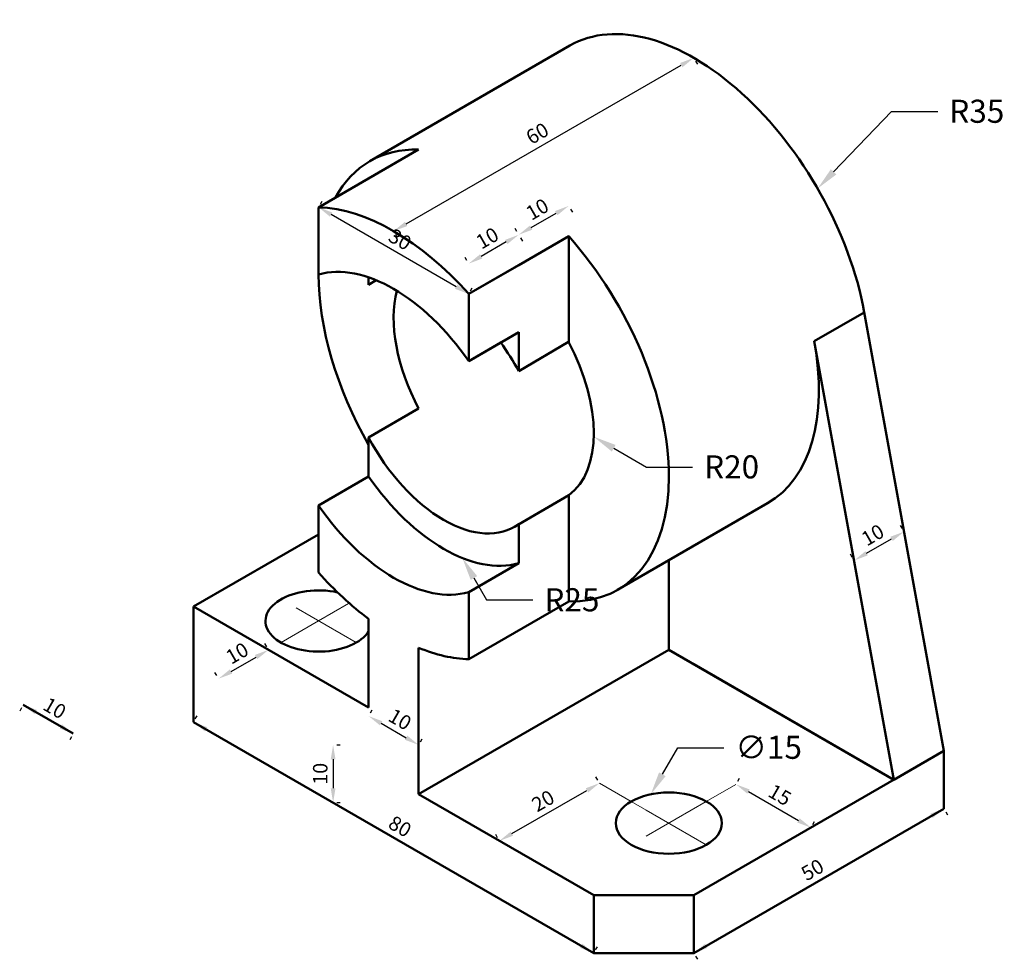
# Model space of a CAD drawing. Units: millimetres. Extents: x 7448 to 7618, y 7987 to 8150.
import ezdxf
from ezdxf import colors
from ezdxf.entities.mleader import LeaderData, LeaderLine
from ezdxf.math import Vec2, Vec3

# ---------------------------------------------------------------- set-up
doc = ezdxf.new("R2010")
doc.units = ezdxf.units.MM
doc.linetypes.add('ACAD_ISO02W100', pattern=[15, 12, -3])
for name, color, linetype, lineweight in [('M-CNTR', 1, 'ACAD_ISO02W100', 18), ('M-CONS', 8, 'ACAD_ISO02W100', 13), ('M-DIMS', 2, 'Continuous', 25), ('M-OUTL', 7, 'Continuous', 50), ('M-TEXT', 3, 'Continuous', 25)]:
    doc.layers.add(name, color=color, linetype=linetype, lineweight=lineweight)
doc.styles.get("Standard").update_dxf_attribs({"font": 'arial.ttf'})
doc.dimstyles.new('ISO-25', dxfattribs={"dimtxt": 2.5, "dimasz": 2.5, "dimexe": 1.25, "dimexo": 0.625, "dimtad": 1, "dimtxsty": 'Standard', "dimcen": 2.5, "dimadec": 0, "dimazin": 0, "dimtfac": 1, "dimtmove": 0, "dimatfit": 3, "dimfxl": 1, "dimarcsym": 0})

# ---------------------------------------------------------------- blocks, each defined once
blk = doc.blocks.new('*D1')
at = {"layer": 'Defpoints', "color": 0, "transparency": 16777216}
for p in [(7502.21, 8024.15), (7502.21, 8014.15), (7502.21, 8014.15)]:
    blk.add_point(p, dxfattribs=at)
at = {"layer": 'M-DIMS', "color": 0, "lineweight": -2, "transparency": 16777216}
for p, q in [((7502.84, 8024.15), (7503.46, 8024.15)), ((7502.21, 8021.65), (7502.21, 8016.65)), ((7502.84, 8014.15), (7503.46, 8014.15))]:
    blk.add_line(p, q, dxfattribs=at)
at = {"layer": 'M-DIMS', "color": 0, "transparency": 16777216}
for points in [[(7501.8, 8021.65), (7502.63, 8021.65), (7502.21, 8024.15)], [(7501.8, 8016.65), (7502.63, 8016.65), (7502.21, 8014.15)]]:
    blk.add_solid(points, dxfattribs=at)
at = {"layer": 'M-DIMS', "color": 0, "transparency": 16777216, "insert": (7500.31, 8019.15), "char_height": 2.5, "attachment_point": 5, "rotation": 90}
blk.add_mtext('10', dxfattribs=at)
blk = doc.blocks.new('*D2')
at = {"layer": 'Defpoints', "color": 0, "transparency": 16777216}
for p in [(7508.36, 8029.14), (7517.02, 8024.14), (7517.02, 8024.14)]:
    blk.add_point(p, dxfattribs=at)
at = {"layer": 'M-DIMS', "color": 0, "lineweight": -2, "transparency": 16777216}
for p, q in [((7508.67, 8029.68), (7508.98, 8030.22)), ((7510.52, 8027.89), (7514.85, 8025.39)), ((7517.33, 8024.68), (7517.64, 8025.22))]:
    blk.add_line(p, q, dxfattribs=at)
at = {"layer": 'M-DIMS', "color": 0, "transparency": 16777216}
for points in [[(7510.73, 8028.25), (7510.32, 8027.53), (7508.36, 8029.14)], [(7515.06, 8025.75), (7514.65, 8025.03), (7517.02, 8024.14)]]:
    blk.add_solid(points, dxfattribs=at)
at = {"layer": 'M-DIMS', "color": 0, "transparency": 16777216, "insert": (7513.64, 8028.29), "char_height": 2.5, "attachment_point": 5, "rotation": 330}
blk.add_mtext('10', dxfattribs=at)
blk = doc.blocks.new('*D3')
at = {"layer": 'Defpoints', "color": 0, "transparency": 16777216}
for p in [(7543, 8117.48), (7543, 8117.48), (7534.34, 8112.48)]:
    blk.add_point(p, dxfattribs=at)
at = {"layer": 'M-DIMS', "color": 0, "lineweight": -2, "transparency": 16777216}
for p, q in [((7543.31, 8116.93), (7543.63, 8116.39)), ((7536.51, 8113.73), (7540.84, 8116.23)), ((7534.65, 8111.93), (7534.97, 8111.39))]:
    blk.add_line(p, q, dxfattribs=at)
at = {"layer": 'M-DIMS', "color": 0, "transparency": 16777216}
for points in [[(7540.63, 8116.59), (7541.04, 8115.86), (7543, 8117.48)], [(7536.3, 8114.09), (7536.71, 8113.36), (7534.34, 8112.48)]]:
    blk.add_solid(points, dxfattribs=at)
at = {"layer": 'M-DIMS', "color": 0, "transparency": 16777216, "insert": (7537.72, 8116.62), "char_height": 2.5, "attachment_point": 5, "rotation": 30}
blk.add_mtext('10', dxfattribs=at)
blk = doc.blocks.new('*D4')
at = {"layer": 'Defpoints', "color": 0, "transparency": 16777216}
for p in [(7534.34, 8112.48), (7525.68, 8107.48), (7525.68, 8107.48)]:
    blk.add_point(p, dxfattribs=at)
at = {"layer": 'M-DIMS', "color": 0, "lineweight": -2, "transparency": 16777216}
for p, q in [((7534.03, 8113.02), (7533.72, 8113.56)), ((7532.18, 8111.23), (7527.84, 8108.73)), ((7525.37, 8108.02), (7525.05, 8108.56))]:
    blk.add_line(p, q, dxfattribs=at)
at = {"layer": 'M-DIMS', "color": 0, "transparency": 16777216}
for points in [[(7531.97, 8111.59), (7532.38, 8110.86), (7534.34, 8112.48)], [(7527.64, 8109.09), (7528.05, 8108.36), (7525.68, 8107.48)]]:
    blk.add_solid(points, dxfattribs=at)
at = {"layer": 'M-DIMS', "color": 0, "transparency": 16777216, "insert": (7529.06, 8111.62), "char_height": 2.5, "attachment_point": 5, "rotation": 30}
blk.add_mtext('10', dxfattribs=at)
blk = doc.blocks.new('*D5')
at = {"layer": 'Defpoints', "color": 0, "transparency": 16777216}
for p in [(7564.65, 8143.11), (7564.65, 8143.11), (7512.69, 8113.11)]:
    blk.add_point(p, dxfattribs=at)
at = {"layer": 'M-DIMS', "color": 0, "lineweight": -2, "transparency": 16777216}
for p, q in [((7564.96, 8142.56), (7565.28, 8142.02)), ((7514.85, 8114.36), (7562.49, 8141.86)), ((7513, 8112.56), (7513.31, 8112.02))]:
    blk.add_line(p, q, dxfattribs=at)
at = {"layer": 'M-DIMS', "color": 0, "transparency": 16777216}
for points in [[(7562.28, 8142.22), (7562.69, 8141.49), (7564.65, 8143.11)], [(7514.65, 8114.72), (7515.06, 8113.99), (7512.69, 8113.11)]]:
    blk.add_solid(points, dxfattribs=at)
at = {"layer": 'M-DIMS', "color": 0, "transparency": 16777216, "insert": (7537.72, 8129.75), "char_height": 2.5, "attachment_point": 5, "rotation": 30}
blk.add_mtext('60', dxfattribs=at)
blk = doc.blocks.new('*D6')
at = {"layer": 'Defpoints', "color": 0, "transparency": 16777216}
for p in [(7601.06, 8061.08), (7601.06, 8061.08), (7592.4, 8056.08)]:
    blk.add_point(p, dxfattribs=at)
at = {"layer": 'M-DIMS', "color": 0, "lineweight": -2, "transparency": 16777216}
for p, q in [((7600.75, 8061.62), (7600.43, 8062.16)), ((7594.56, 8057.33), (7598.89, 8059.83)), ((7592.09, 8056.62), (7591.77, 8057.16))]:
    blk.add_line(p, q, dxfattribs=at)
at = {"layer": 'M-DIMS', "color": 0, "transparency": 16777216}
for points in [[(7598.68, 8060.19), (7599.1, 8059.47), (7601.06, 8061.08)], [(7594.35, 8057.69), (7594.77, 8056.97), (7592.4, 8056.08)]]:
    blk.add_solid(points, dxfattribs=at)
at = {"layer": 'M-DIMS', "color": 0, "transparency": 16777216, "insert": (7595.78, 8060.22), "char_height": 2.5, "attachment_point": 5, "rotation": 30}
blk.add_mtext('10', dxfattribs=at)
blk = doc.blocks.new('*D7')
at = {"layer": 'Defpoints', "color": 0, "transparency": 16777216}
for p in [(7491.04, 8040.61), (7491.04, 8040.61), (7482.38, 8035.61)]:
    blk.add_point(p, dxfattribs=at)
at = {"layer": 'M-DIMS', "color": 0, "lineweight": -2, "transparency": 16777216}
for p, q in [((7490.73, 8041.15), (7490.41, 8041.69)), ((7484.54, 8036.86), (7488.87, 8039.36)), ((7482.07, 8036.15), (7481.75, 8036.69))]:
    blk.add_line(p, q, dxfattribs=at)
at = {"layer": 'M-DIMS', "color": 0, "transparency": 16777216}
for points in [[(7488.67, 8039.72), (7489.08, 8038.99), (7491.04, 8040.61)], [(7484.34, 8037.22), (7484.75, 8036.49), (7482.38, 8035.61)]]:
    blk.add_solid(points, dxfattribs=at)
at = {"layer": 'M-DIMS', "color": 0, "transparency": 16777216, "insert": (7485.76, 8039.75), "char_height": 2.5, "attachment_point": 5, "rotation": 30}
blk.add_mtext('10', dxfattribs=at)
blk = doc.blocks.new('*D8')
at = {"layer": 'Defpoints', "color": 0, "transparency": 16777216}
for p in [(7548.32, 8017.53), (7548.32, 8017.53), (7531, 8007.53)]:
    blk.add_point(p, dxfattribs=at)
at = {"layer": 'M-DIMS', "color": 0, "lineweight": -2, "transparency": 16777216}
for p, q in [((7548.01, 8018.07), (7547.7, 8018.61)), ((7533.17, 8008.78), (7546.16, 8016.28)), ((7530.69, 8008.07), (7530.38, 8008.61))]:
    blk.add_line(p, q, dxfattribs=at)
at = {"layer": 'M-DIMS', "color": 0, "transparency": 16777216}
for points in [[(7545.95, 8016.64), (7546.37, 8015.92), (7548.32, 8017.53)], [(7532.96, 8009.14), (7533.38, 8008.42), (7531, 8007.53)]]:
    blk.add_solid(points, dxfattribs=at)
at = {"layer": 'M-DIMS', "color": 0, "transparency": 16777216, "insert": (7538.71, 8014.18), "char_height": 2.5, "attachment_point": 5, "rotation": 30}
blk.add_mtext('20', dxfattribs=at)
blk = doc.blocks.new('*D9')
at = {"layer": 'Defpoints', "color": 0, "transparency": 16777216}
for p in [(7571.95, 8017.32), (7584.94, 8009.82), (7584.94, 8009.82)]:
    blk.add_point(p, dxfattribs=at)
at = {"layer": 'M-DIMS', "color": 0, "lineweight": -2, "transparency": 16777216}
for p, q in [((7572.26, 8017.86), (7572.57, 8018.4)), ((7574.11, 8016.07), (7582.77, 8011.07)), ((7585.25, 8010.36), (7585.56, 8010.9))]:
    blk.add_line(p, q, dxfattribs=at)
at = {"layer": 'M-DIMS', "color": 0, "transparency": 16777216}
for points in [[(7574.32, 8016.43), (7573.9, 8015.71), (7571.95, 8017.32)], [(7582.98, 8011.43), (7582.56, 8010.71), (7584.94, 8009.82)]]:
    blk.add_solid(points, dxfattribs=at)
at = {"layer": 'M-DIMS', "color": 0, "transparency": 16777216, "insert": (7579.39, 8015.21), "char_height": 2.5, "attachment_point": 5, "rotation": 330}
blk.add_mtext('15', dxfattribs=at)
blk = doc.blocks.new('*D10')
at = {"layer": 'Defpoints', "color": 0, "transparency": 16777216}
for p in [(7499.7, 8117.23), (7499.7, 8117.23), (7525.68, 8102.23)]:
    blk.add_point(p, dxfattribs=at)
at = {"layer": 'M-DIMS', "color": 0, "lineweight": -2, "transparency": 16777216}
for p, q in [((7500.01, 8117.77), (7500.32, 8118.31)), ((7523.51, 8103.48), (7501.86, 8115.98)), ((7525.99, 8102.77), (7526.3, 8103.31))]:
    blk.add_line(p, q, dxfattribs=at)
at = {"layer": 'M-DIMS', "color": 0, "transparency": 16777216}
for points in [[(7502.07, 8116.34), (7501.66, 8115.62), (7499.7, 8117.23)], [(7523.72, 8103.84), (7523.31, 8103.12), (7525.68, 8102.23)]]:
    blk.add_solid(points, dxfattribs=at)
at = {"layer": 'M-DIMS', "color": 0, "transparency": 16777216, "insert": (7513.64, 8111.38), "char_height": 2.5, "attachment_point": 5, "rotation": 330}
blk.add_mtext('30', dxfattribs=at)
blk = doc.blocks.new('*D11')
at = {"layer": 'Defpoints', "color": 0, "transparency": 16777216}
for p in [(7478.05, 8028.11), (7547.33, 7988.11), (7547.33, 7988.11)]:
    blk.add_point(p, dxfattribs=at)
at = {"layer": 'M-DIMS', "color": 0, "lineweight": -2, "transparency": 16777216}
for p, q in [((7478.36, 8028.65), (7478.67, 8029.19)), ((7480.21, 8026.86), (7545.17, 7989.36)), ((7547.64, 7988.65), (7547.96, 7989.19))]:
    blk.add_line(p, q, dxfattribs=at)
at = {"layer": 'M-DIMS', "color": 0, "transparency": 16777216}
for points in [[(7480.42, 8027.22), (7480.01, 8026.49), (7478.05, 8028.11)], [(7545.37, 7989.72), (7544.96, 7988.99), (7547.33, 7988.11)]]:
    blk.add_solid(points, dxfattribs=at)
at = {"layer": 'M-DIMS', "color": 0, "transparency": 16777216, "insert": (7513.64, 8009.75), "char_height": 2.5, "attachment_point": 5, "rotation": 330}
blk.add_mtext('80', dxfattribs=at)
blk = doc.blocks.new('*D12')
at = {"layer": 'Defpoints', "color": 0, "transparency": 16777216}
for p in [(7607.95, 8013.11), (7564.65, 7988.11), (7564.65, 7988.11)]:
    blk.add_point(p, dxfattribs=at)
at = {"layer": 'M-DIMS', "color": 0, "lineweight": -2, "transparency": 16777216}
for p, q in [((7608.26, 8012.56), (7608.58, 8012.02)), ((7605.79, 8011.86), (7566.82, 7989.36)), ((7564.96, 7987.56), (7565.28, 7987.02))]:
    blk.add_line(p, q, dxfattribs=at)
at = {"layer": 'M-DIMS', "color": 0, "transparency": 16777216}
for points in [[(7605.58, 8012.22), (7606, 8011.49), (7607.95, 8013.11)], [(7566.61, 7989.72), (7567.02, 7988.99), (7564.65, 7988.11)]]:
    blk.add_solid(points, dxfattribs=at)
at = {"layer": 'M-DIMS', "color": 0, "transparency": 16777216, "insert": (7585.35, 8002.25), "char_height": 2.5, "attachment_point": 5, "rotation": 30}
blk.add_mtext('50', dxfattribs=at)
blk = doc.blocks.new('*D13')
at = {"layer": 'Defpoints', "color": 0, "transparency": 16777216}
for p in [(7448.58, 8031.09), (7448.58, 8031.09), (7457.24, 8026.09)]:
    blk.add_point(p, dxfattribs=at)
at = {"layer": 'M-DIMS', "color": 0, "lineweight": -2, "transparency": 16777216}
for p, q in [((7448.27, 8030.55), (7447.96, 8030.01)), ((7455.08, 8027.34), (7450.75, 8029.84)), ((7456.93, 8025.55), (7456.62, 8025.01))]:
    blk.add_line(p, q, dxfattribs=at)
at = {"layer": 'M-DIMS', "color": 0, "transparency": 16777216}
for points in [[(7450.96, 8030.2), (7450.54, 8029.48), (7448.58, 8031.09)], [(7455.29, 8027.7), (7454.87, 8026.98), (7457.24, 8026.09)]]:
    blk.add_solid(points, dxfattribs=at)
at = {"layer": 'M-DIMS', "color": 0, "transparency": 16777216, "insert": (7453.86, 8030.24), "char_height": 2.5, "attachment_point": 5, "rotation": 330}
blk.add_mtext('10', dxfattribs=at)

msp = doc.modelspace()

# ---------------------------------------------------------------- linework, layer by layer
at = {"layer": 'M-CNTR'}
for p, q in [((7506.194, 8041.855), (7493.204, 8049.355)), ((7504.898, 8048.607), (7499.699, 8045.605)), ((7499.699, 8045.605), (7493.204, 8041.855)), ((7553.826, 8014.355), (7548.324, 8017.532)), ((7566.816, 8014.355), (7571.948, 8017.318)), ((7566.816, 8014.355), (7553.826, 8006.855)), ((7560.321, 8010.605), (7553.826, 8014.355)), ((7556.397, 8012.871), (7566.816, 8006.855))]:
    msp.add_line(p, q, dxfattribs=at)
at = {"layer": 'M-CONS'}
msp.add_line((7478.048, 8048.105), (7491.039, 8040.605), dxfattribs=at)
at = {"layer": 'M-OUTL'}
for p, q in [((7508.577, 8125.228), (7543.218, 8145.228)), ((7543.218, 8145.228), (7508.577, 8125.228)), ((7499.699, 8117.228), (7517.02, 8127.228)), ((7499.699, 8117.228), (7499.699, 8105.605)), ((7525.68, 8102.228), (7543, 8112.228)), ((7534.34, 8107.228), (7543, 8112.228)), ((7543, 8112.228), (7543, 8093.834)), ((7525.68, 8102.228), (7534.34, 8107.228)), ((7508.36, 8105.1), (7508.36, 8103.834)), ((7508.36, 8103.834), (7509.684, 8104.598)), ((7525.68, 8102.228), (7525.68, 8095.24)), ((7525.68, 8102.228), (7525.68, 8090.605)), ((7585.505, 8094.04), (7594.165, 8099.04)), ((7607.952, 8023.105), (7594.163, 8099.048)), ((7525.68, 8090.605), (7534.34, 8095.605)), ((7534.34, 8095.605), (7534.34, 8088.834)), ((7534.34, 8095.605), (7534.34, 8088.834)), ((7525.68, 8090.605), (7531.239, 8093.815)), ((7542.951, 8093.926), (7534.34, 8088.834)), ((7542.951, 8093.926), (7543, 8093.954)), ((7599.292, 8018.105), (7585.503, 8094.048)), ((7508.359, 8077.377), (7517.02, 8082.377)), ((7508.359, 8070.605), (7508.359, 8077.377)), ((7499.699, 8065.605), (7508.359, 8070.605)), ((7560.321, 8070.605), (7560.321, 8070.788)), ((7533.597, 8061.892), (7543, 8067.377)), ((7543, 8048.983), (7543, 8067.377)), ((7499.699, 8065.605), (7499.699, 8053.983)), ((7551.443, 8050.982), (7577.424, 8065.982)), ((7534.34, 8055.605), (7534.34, 8062.377)), ((7478.048, 8048.105), (7499.699, 8060.605)), ((7525.68, 8050.605), (7534.34, 8055.605)), ((7560.321, 8040.605), (7560.321, 8056.108)), ((7525.68, 8050.605), (7525.68, 8038.983)), ((7525.68, 8038.983), (7543, 8048.983)), ((7525.68, 8038.983), (7543, 8048.983)), ((7478.048, 8028.105), (7478.048, 8048.105)), ((7508.36, 8030.605), (7478.049, 8048.105)), ((7508.36, 8030.605), (7508.36, 8045.964)), ((7517.02, 8015.605), (7517.02, 8040.964)), ((7517.02, 8015.605), (7560.321, 8040.605)), ((7517.02, 8015.605), (7560.321, 8040.605)), ((7599.292, 8018.105), (7560.321, 8040.605)), ((7478.048, 8028.105), (7478.048, 8038.105)), ((7599.292, 8018.105), (7564.651, 8038.105)), ((7457.244, 8026.094), (7448.584, 8031.094)), ((7478.048, 8028.105), (7547.33, 7988.105)), ((7547.33, 7988.105), (7478.048, 8028.105)), ((7564.651, 7998.105), (7607.952, 8023.105)), ((7607.952, 8023.105), (7599.292, 8018.105)), ((7607.952, 8023.105), (7599.292, 8018.105)), ((7607.952, 8023.105), (7599.292, 8018.105)), ((7607.952, 8023.105), (7599.292, 8018.105)), ((7607.952, 8023.105), (7607.952, 8013.105)), ((7517.02, 8015.605), (7547.33, 7998.105)), ((7564.651, 7988.105), (7607.952, 8013.105)), ((7547.33, 7998.105), (7564.651, 7998.105)), ((7547.33, 7998.105), (7547.33, 7988.105)), ((7564.651, 7998.105), (7564.651, 7988.105)), ((7554.651, 7988.105), (7547.33, 7988.105)), ((7564.651, 7988.105), (7554.651, 7988.105))]:
    msp.add_line(p, q, dxfattribs=at)
for centre, major_axis, start_param, end_param in [((7564.651, 8108.105), (21.433, -37.123), 7.2986503, 9.424778), ((7530.01, 8088.105), (21.433, -37.123), 9.0822908, 9.7672651), ((7512.689, 8078.105), (21.433, -37.123), 8.1964688, 9.0822908), ((7530.01, 8088.105), (21.433, -37.123), 5.9406982, 8.1964688), ((7530.01, 8088.105), (21.433, -37.123), 5.9406982, 8.1964688), ((7512.689, 8078.105), (15.309, -26.517), 7.9958787, 9.2828809), ((7530.01, 8088.105), (21.433, -37.123), 10.2101761, 10.9853695), ((7521.35, 8083.105), (12.247, -21.213), 3.1415927, 3.2042566), ((7530.01, 8088.105), (12.247, -21.213), 3.6747245, 4.6497251), ((7521.35, 8083.105), (12.247, -21.213), 1.5081324, 1.7485069), ((7530.01, 8088.105), (12.247, -21.213), 1.5081324, 1.512392), ((7530.01, 8088.105), (12.247, -21.213), 6.3458492, 7.7955773), ((7555.991, 8103.105), (21.433, -37.123), 6.2831853, 7.2986503), ((7521.35, 8083.105), (12.247, -21.213), 4.6497251, 6.3458492), ((7521.35, 8083.105), (12.247, -21.213), 4.6497251, 6.3458492), ((7521.35, 8083.105), (12.247, -21.213), 4.6497251, 6.3458492), ((7521.35, 8083.105), (12.247, -21.213), 4.6497251, 6.3458492), ((7521.35, 8083.105), (15.309, -26.517), 4.854286, 6.1412883), ((7521.35, 8083.105), (15.309, -26.517), 4.854286, 6.1412883), ((7512.689, 8078.105), (15.309, -26.517), 4.854286, 6.1412883), ((7512.689, 8078.105), (15.309, -26.517), 4.854286, 6.1412883), ((7512.689, 8078.105), (21.433, -37.123), 11.3380614, 11.6376249), ((7512.689, 8078.105), (21.433, -37.123), 5.0548761, 5.3544396), ((7499.699, 8045.605), (-9.186, 0), 4.3476754, 9.0849411), ((7512.689, 8078.105), (21.433, -37.123), 5.6411347, 5.9406982), ((7512.689, 8078.105), (21.433, -37.123), 5.6411347, 5.9406982)]:
    msp.add_ellipse(centre, major_axis=major_axis, ratio=0.5773503, start_param=start_param, end_param=end_param, dxfattribs=at)
msp.add_ellipse((7560.321, 8010.605), major_axis=(-9.186, 0), ratio=0.5773503, dxfattribs=at)

# ---------------------------------------------------------------- dimensions: what is measured, and where the dimension line sits
at = {"layer": 'M-DIMS'}
for p1, p2, picture, middle in [((7512.689, 8113.105), (7564.651, 8143.105), '*D5', (7537.72, 8129.752)), ((7534.34, 8112.475), (7543, 8117.475), '*D3', (7537.72, 8116.622)), ((7534.34, 8112.475), (7525.68, 8107.475), '*D4', (7529.059, 8111.622)), ((7592.398, 8056.077), (7601.058, 8061.077), '*D6', (7595.777, 8060.223)), ((7482.379, 8035.605), (7491.039, 8040.605), '*D7', (7485.758, 8039.752)), ((7508.359, 8029.14), (7517.02, 8024.14), '*D2', (7513.64, 8028.287)), ((7502.213, 8024.154), (7502.213, 8014.154), '*D1', (7500.311, 8019.154)), ((7531.003, 8007.532), (7548.324, 8017.532), '*D8', (7538.713, 8014.179)), ((7571.948, 8017.318), (7584.938, 8009.818), '*D9', (7579.394, 8015.215))]:
    dim = msp.add_aligned_dim(p1=p1, p2=p2, distance=0, dimstyle='ISO-25', override={"dimclrd": 0, "dimclre": 0, "dimclrt": 0}, dxfattribs=at)
    dim.commit()
    dim.dimension.update_dxf_attribs({"geometry": picture, "text_midpoint": middle})
for base, p1, p2, angle, picture, middle in [((7499.699, 8117.228), (7525.68, 8102.228), (7499.699, 8117.228), 150, '*D10', (7513.641, 8111.376)), ((7448.584, 8031.094), (7457.244, 8026.094), (7448.584, 8031.094), 150, '*D13', (7453.865, 8030.241)), ((7547.33, 7988.105), (7478.048, 8028.105), (7547.33, 7988.105), 330, '*D11', (7513.64, 8009.752)), ((7564.651, 7988.105), (7607.952, 8013.105), (7564.651, 7988.105), 210, '*D12', (7585.351, 8002.252))]:
    dim = msp.add_linear_dim(base=base, p1=p1, p2=p2, angle=angle, dimstyle='ISO-25', override={"dimrnd": 0}, dxfattribs=at)
    dim.commit()
    dim.dimension.update_dxf_attribs({"geometry": picture, "text_midpoint": middle})

# ---------------------------------------------------------------- leaders
at = {"layer": 'M-TEXT'}
ml = msp.add_multileader_mtext('Standard', dxfattribs=at)
ml.set_content('R35', color=256)
ml.set_leader_properties()
ml.build(insert=Vec2(0, 0))
ctx = ml.context
ctx.base_point, ctx.plane_origin = Vec3(7606.877, 8133.83), Vec3(7586.084, 8120.48)
notes = []
notes.append((ctx, [(0, (1, 1, 0), (7598.877, 8133.83), (1, 0), 8, [(0, [(7586.084, 8120.48)], 0, [])])]))
ctx.mtext.insert, ctx.mtext.flow_direction = Vec3(7608.877, 8135.866), 5
ml = msp.add_multileader_mtext('Standard', dxfattribs=at)
ml.set_content('R20', color=256)
ml.set_leader_properties()
ml.build(insert=Vec2(0, 0))
ctx = ml.context
ctx.base_point, ctx.plane_origin = Vec3(7564.434, 8072.253), Vec3(7547.323, 8077.514)
notes.append((ctx, [(0, (1, 1, 0), (7556.434, 8072.253), (1, 0), 8, [(0, [(7547.323, 8077.514)], 0, [])])]))
ctx.mtext.insert, ctx.mtext.flow_direction = Vec3(7566.434, 8074.288), 5
ml = msp.add_multileader_mtext('Standard', dxfattribs=at)
ml.set_content('R25', color=256)
ml.set_leader_properties()
ml.build(insert=Vec2(0, 0))
ctx = ml.context
ctx.base_point, ctx.plane_origin = Vec3(7536.791, 8049.242), Vec3(7524.592, 8056.515)
notes.append((ctx, [(0, (1, 1, 0), (7528.791, 8049.242), (1, 0), 8, [(0, [(7524.592, 8056.515)], 0, [])])]))
ctx.mtext.insert, ctx.mtext.flow_direction = Vec3(7538.791, 8051.276), 5
ml = msp.add_multileader_mtext('Standard', dxfattribs=at)
ml.set_content('∅15', color=256)
ml.set_leader_properties()
ml.build(insert=Vec2(0, 0))
ctx = ml.context
ctx.base_point, ctx.plane_origin = Vec3(7569.858, 8023.657), Vec3(7557.203, 8015.594)
notes.append((ctx, [(0, (1, 1, 0), (7561.858, 8023.657), (1, 0), 8, [(0, [(7557.203, 8015.594)], 0, [])])]))
ctx.mtext.insert, ctx.mtext.flow_direction = Vec3(7571.858, 8025.737), 5
for ctx, leaders in notes:
    for number, flags, end, landing, length, lines in leaders:
        leader = LeaderData()
        leader.index, (leader.has_last_leader_line, leader.has_dogleg_vector, leader.attachment_direction) = number, flags
        leader.last_leader_point, leader.dogleg_vector, leader.dogleg_length = Vec3(end), Vec3(landing), length
        for number, points, colour, breaks in lines:
            line = LeaderLine()
            line.index, line.vertices, line.color, line.breaks = number, Vec3.list(points), colors.encode_raw_color(colour), breaks
            leader.lines.append(line)
        ctx.leaders.append(leader)

doc.saveas('drawing.dxf')
